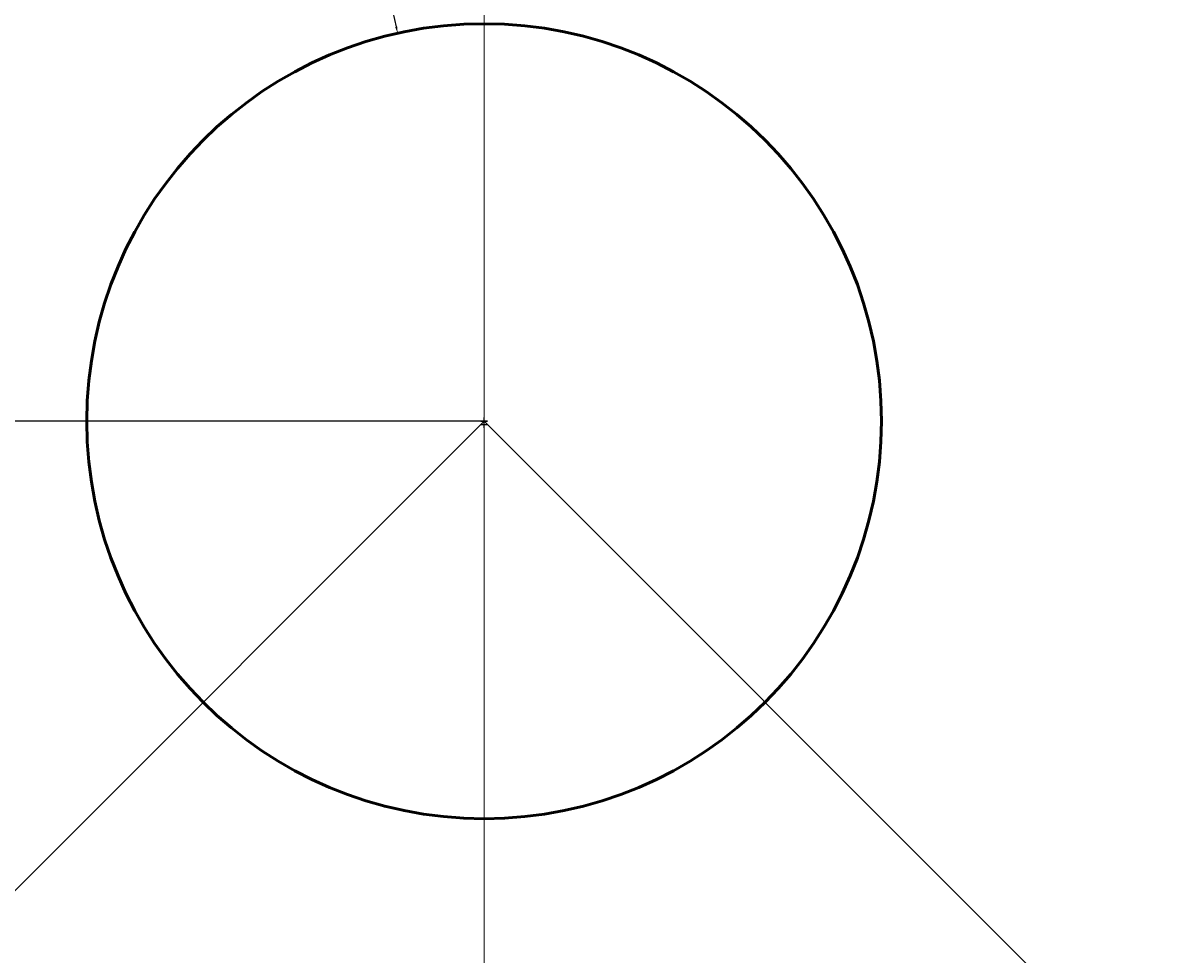
# Model space of a CAD drawing. Units: millimetres. Extents: x -53 to 92, y -147 to 37.
# Tile 7 of 16: x 6 to 38, y -69 to -43. Entities that reach past the tile are written whole.
import ezdxf

# ---------------------------------------------------------------- set-up
doc = ezdxf.new("R2010")
doc.units = ezdxf.units.MM
doc.header["$MEASUREMENT"] = 0
doc.linetypes.add('CENTER', pattern=[50.8, 31.75, -6.35, 6.35, -6.35])
for name, color, linetype, lineweight in [('M-CNTR', 4, 'CENTER', 18), ('M-DIMS', 2, 'Continuous', 25), ('M-OUTL', 7, 'Continuous', 50)]:
    doc.layers.add(name, color=color, linetype=linetype, lineweight=lineweight)
doc.styles.get("Standard").update_dxf_attribs({"font": 'arial.ttf'})
doc.dimstyles.get("Standard").update_dxf_attribs({"dimtxt": 0.18, "dimasz": 0.18, "dimexe": 0.18, "dimexo": 0.0625, "dimgap": 0.09, "dimtad": 0, "dimtih": 1, "dimtoh": 1, "dimdec": 4, "dimzin": 0, "dimdsep": 46, "dimtxsty": 'Standard', "dimcen": 0.09, "dimadec": 0, "dimazin": 0, "dimtfac": 1, "dimtdec": 4, "dimtofl": 0, "dimtmove": 0, "dimatfit": 3, "dimfxl": 1, "dimtolj": 1, "dimtzin": 0, "dimarcsym": 0})

# ---------------------------------------------------------------- blocks, each defined once
blk = doc.blocks.new('*D7')
at = {"layer": 'Defpoints', "color": 0, "transparency": 16777216}
for p in [(9.445, -3.88), (-44.321, -53.98), (18.956, -53.98)]:
    blk.add_point(p, dxfattribs=at)
at = {"layer": 'M-DIMS', "color": 0, "lineweight": -2, "transparency": 16777216}
for p, q in [((9.382, -3.88), (-44.501, -3.88)), ((-44.321, -4.06), (-44.321, -27.308)), ((-44.321, -53.8), (-44.321, -30.552)), ((18.894, -53.98), (-44.501, -53.98))]:
    blk.add_line(p, q, dxfattribs=at)
at = {"layer": 'M-DIMS', "color": 0, "transparency": 16777216}
for points in [[(-44.351, -4.06), (-44.291, -4.06), (-44.321, -3.88)], [(-44.351, -53.8), (-44.291, -53.8), (-44.321, -53.98)]]:
    blk.add_solid(points, dxfattribs=at)
at = {"layer": 'M-DIMS', "color": 0, "transparency": 16777216, "insert": (-44.321, -28.93), "char_height": 0.18, "attachment_point": 5}
blk.add_mtext('\\A1;{\\H16.66667x;50}', dxfattribs=at)
blk = doc.blocks.new('*D10')
at = {"layer": 'Defpoints', "color": 0, "transparency": 16777216}
for p in [(64.593, -18.184), (-26.68, -89.776)]:
    blk.add_point(p, dxfattribs=at)
at = {"layer": 'M-DIMS', "color": 0, "lineweight": -2, "transparency": 16777216}
for p, q in [((77.384, -8.151), (64.734, -18.073)), ((77.564, -8.151), (77.384, -8.151)), ((18.866, -53.98), (19.046, -53.98)), ((18.956, -54.07), (18.956, -53.89))]:
    blk.add_line(p, q, dxfattribs=at)
at = {"layer": 'M-DIMS', "color": 0, "transparency": 16777216}
blk.add_solid([(64.716, -18.05), (64.753, -18.097), (64.593, -18.184)], dxfattribs=at)
at = {"layer": 'M-DIMS', "color": 0, "transparency": 16777216, "insert": (82.599, -8.151), "char_height": 0.18, "attachment_point": 5}
blk.add_mtext('\\A1;{\\H16.66667x;%%C116}', dxfattribs=at)
blk = doc.blocks.new('*D12')
at = {"layer": 'Defpoints', "color": 0, "transparency": 16777216}
for p in [(18.956, -54.07), (37.579, -89.471)]:
    blk.add_point(p, dxfattribs=at)
at = {"layer": 'M-DIMS', "color": 0, "lineweight": -2, "transparency": 16777216}
for p, q in [((30.294, -75.965), (30.474, -75.965)), ((30.474, -75.965), (37.495, -89.311))]:
    blk.add_line(p, q, dxfattribs=at)
at = {"layer": 'M-DIMS', "color": 0, "transparency": 16777216}
blk.add_solid([(37.522, -89.297), (37.469, -89.325), (37.579, -89.471)], dxfattribs=at)
at = {"layer": 'M-DIMS', "color": 0, "transparency": 16777216, "insert": (26.625, -75.965), "char_height": 0.18, "attachment_point": 5}
blk.add_mtext('\\A1;{\\H16.66667x;R40}', dxfattribs=at)
blk = doc.blocks.new('*D13')
at = {"layer": 'Defpoints', "color": 0, "transparency": 16777216}
for p in [(16.562, -43.244), (21.351, -64.716)]:
    blk.add_point(p, dxfattribs=at)
at = {"layer": 'M-DIMS', "color": 0, "lineweight": -2, "transparency": 16777216}
for p, q in [((14.214, -33.523), (14.394, -33.523)), ((14.394, -33.523), (16.523, -43.068)), ((18.866, -53.98), (19.046, -53.98)), ((18.956, -54.07), (18.956, -53.89))]:
    blk.add_line(p, q, dxfattribs=at)
at = {"layer": 'M-DIMS', "color": 0, "transparency": 16777216}
blk.add_solid([(16.552, -43.062), (16.494, -43.075), (16.562, -43.244)], dxfattribs=at)
at = {"layer": 'M-DIMS', "color": 0, "transparency": 16777216, "insert": (10.359, -33.523), "char_height": 0.18, "attachment_point": 5}
blk.add_mtext('\\A1;{\\H16.66667x;%%C22}', dxfattribs=at)
blk = doc.blocks.new('*D17')
at = {"layer": 'Defpoints', "color": 0, "transparency": 16777216}
for p in [(-46.81, 25.909), (28.564, 25.909), (18.165, -111.975)]:
    blk.add_point(p, dxfattribs=at)
at = {"layer": 'M-DIMS', "color": 0, "lineweight": -2, "transparency": 16777216}
for p, q in [((28.502, 25.909), (-46.99, 25.909)), ((-46.81, 25.729), (-46.81, -42.851)), ((-46.81, -111.795), (-46.81, -43.215)), ((18.102, -111.975), (-46.99, -111.975))]:
    blk.add_line(p, q, dxfattribs=at)
at = {"layer": 'M-DIMS', "color": 0, "transparency": 16777216}
for points in [[(-46.84, 25.729), (-46.78, 25.729), (-46.81, 25.909)], [(-46.84, -111.795), (-46.78, -111.795), (-46.81, -111.975)]]:
    blk.add_solid(points, dxfattribs=at)
at = {"layer": 'M-DIMS', "color": 0, "transparency": 16777216, "insert": (-46.81, -43.033), "char_height": 0.18, "attachment_point": 5}
blk.add_mtext('\\A1;137.88', dxfattribs=at)
blk = doc.blocks.new('*D18')
at = {"layer": 'Defpoints', "color": 0, "transparency": 16777216}
for p in [(19.753, 4.014), (18.16, -111.975)]:
    blk.add_point(p, dxfattribs=at)
at = {"layer": 'M-DIMS', "color": 0, "lineweight": -2, "transparency": 16777216}
for p, q in [((18.866, -53.98), (19.046, -53.98)), ((18.956, -54.07), (18.956, -53.89)), ((17.682, -146.771), (18.158, -112.155)), ((17.502, -146.771), (17.682, -146.771))]:
    blk.add_line(p, q, dxfattribs=at)
at = {"layer": 'M-DIMS', "color": 0, "transparency": 16777216}
blk.add_solid([(18.128, -112.154), (18.188, -112.155), (18.16, -111.975)], dxfattribs=at)
at = {"layer": 'M-DIMS', "color": 0, "transparency": 16777216, "insert": (17.115, -146.771), "char_height": 0.18, "attachment_point": 5}
blk.add_mtext('\\A1;∅116', dxfattribs=at)
blk = doc.blocks.new('*D23')
at = {"layer": 'Defpoints', "color": 0, "transparency": 16777216}
for p in [(18.956, -54.07), (18.954, -94.07)]:
    blk.add_point(p, dxfattribs=at)
at = {"layer": 'M-DIMS', "color": 0, "lineweight": -2, "transparency": 16777216}
for p, q in [((18.956, -54.16), (18.956, -53.98)), ((18.866, -54.07), (19.046, -54.07)), ((18.953, -118.07), (18.954, -94.25)), ((18.773, -118.07), (18.953, -118.07))]:
    blk.add_line(p, q, dxfattribs=at)
at = {"layer": 'M-DIMS', "color": 0, "transparency": 16777216}
blk.add_solid([(18.924, -94.25), (18.984, -94.25), (18.954, -94.07)], dxfattribs=at)
at = {"layer": 'M-DIMS', "color": 0, "transparency": 16777216, "insert": (18.468, -118.07), "char_height": 0.18, "attachment_point": 5}
blk.add_mtext('\\A1;R40', dxfattribs=at)
blk = doc.blocks.new('*D24')
at = {"layer": 'Defpoints', "color": 0, "transparency": 16777216}
for p in [(18.956, -53.969), (2.002, -101.015)]:
    blk.add_point(p, dxfattribs=at)
at = {"layer": 'M-DIMS', "color": 0, "lineweight": -2, "transparency": 16777216}
for p, q in [((18.866, -53.969), (19.046, -53.969)), ((18.956, -54.059), (18.956, -53.879)), ((-8.171, -129.243), (1.941, -101.184)), ((-8.351, -129.243), (-8.171, -129.243))]:
    blk.add_line(p, q, dxfattribs=at)
at = {"layer": 'M-DIMS', "color": 0, "transparency": 16777216}
blk.add_solid([(1.912, -101.174), (1.969, -101.195), (2.002, -101.015)], dxfattribs=at)
at = {"layer": 'M-DIMS', "color": 0, "transparency": 16777216, "insert": (-8.813, -129.243), "char_height": 0.18, "attachment_point": 5}
blk.add_mtext('\\A1;R50.01', dxfattribs=at)

msp = doc.modelspace()

# ---------------------------------------------------------------- linework, layer by layer
at = {"layer": 'M-CNTR'}
for p, q in [((18.95638, -54.07007), (18.95638, -15.58399)), ((18.95638, -53.98007), (-27.00556, -99.94201)), ((18.95638, -53.98007), (64.91832, -99.94201)), ((18.95638, -53.98007), (18.95638, -130.36235))]:
    msp.add_line(p, q, dxfattribs=at)
msp.add_arc((18.95638, -54.07007), 40, 187.365915, 352.627832, dxfattribs=at)
at = {"layer": 'M-OUTL'}
msp.add_circle((18.95638, -53.98007), 11, dxfattribs=at)
msp.add_arc((18.95638, -53.98007), 58, 108.3895553, 70.0459142, dxfattribs=at)

# ---------------------------------------------------------------- dimensions: what is measured, and where the dimension line sits
at = {"layer": 'M-DIMS'}
dim = msp.add_linear_dim(base=(-46.8103, 25.90924), p1=(18.16452, -111.97467), p2=(28.56407, 25.90924), angle=90, dimstyle='Standard', override={"dimdec": 2, "dimlfac": 1, "dimrnd": 0, "dimzin": 0, "dimdsep": 46, "dimlunit": 2}, dxfattribs=at)
dim.commit()
dim.dimension.update_dxf_attribs({"geometry": '*D17', "text_midpoint": (-46.8103, -43.03271)})
dim = msp.add_diameter_dim_2p(p1=(19.75275, 4.01446), p2=(18.16001, -111.9746), dimstyle='Standard', override={"dimdec": 0, "dimlfac": 1, "dimrnd": 0, "dimzin": 0, "dimdsep": 46, "dimlunit": 2}, dxfattribs=at)
dim.commit()
dim.dimension.update_dxf_attribs({"geometry": '*D18', "text_midpoint": (17.11548, -146.77132), "dimtype": 163})
dim = msp.add_linear_dim(base=(-44.32095, -53.98007), p1=(9.44461, -3.87977), p2=(18.95638, -53.98007), angle=90, text='{\\H16.66667x;50}', dimstyle='Standard', override={"dimclrd": 0, "dimclre": 0, "dimclrt": 0}, dxfattribs=at)
dim.commit()
dim.dimension.update_dxf_attribs({"geometry": '*D7', "text_midpoint": (-44.32095, -28.92992)})
for p1, p2, text, picture, middle in [((-26.67986, -89.77579), (64.59262, -18.18435), '{\\H16.66667x;%%C116}', '*D10', (82.59889, -8.15132)), ((21.35078, -64.71631), (16.56198, -43.24383), '{\\H16.66667x;%%C22}', '*D13', (10.35867, -33.52288))]:
    dim = msp.add_diameter_dim_2p(p1=p1, p2=p2, text=text, dimstyle='Standard', override={"dimclrd": 0, "dimclre": 0, "dimclrt": 0}, dxfattribs=at)
    dim.commit()
    dim.dimension.update_dxf_attribs({"geometry": picture, "text_midpoint": middle, "dimtype": 163})
for center, mpoint, override, picture, middle in [((18.95621, -53.96903), (2.00175, -101.01516), {"dimdec": 2, "dimlfac": 1, "dimrnd": 0, "dimzin": 0, "dimdsep": 46, "dimlunit": 2}, '*D24', (-8.8134, -129.24283)), ((18.95638, -54.07007), (18.954, -94.07007), {"dimdec": 0, "dimlfac": 1, "dimrnd": 0, "dimzin": 0, "dimdsep": 46, "dimlunit": 2}, '*D23', (18.46782, -118.07007))]:
    dim = msp.add_radius_dim(center=center, mpoint=mpoint, dimstyle='Standard', override=override, dxfattribs=at)
    dim.commit()
    dim.dimension.update_dxf_attribs({"geometry": picture, "text_midpoint": middle, "dimtype": 164})
dim = msp.add_radius_dim(center=(18.95638, -54.07007), mpoint=(37.5792, -89.4705), text='{\\H16.66667x;R40}', dimstyle='Standard', override={"dimclrd": 0, "dimclre": 0, "dimclrt": 0}, dxfattribs=at)
dim.commit()
dim.dimension.update_dxf_attribs({"geometry": '*D12', "text_midpoint": (26.62522, -75.96478), "dimtype": 164})

doc.saveas('drawing.dxf')
